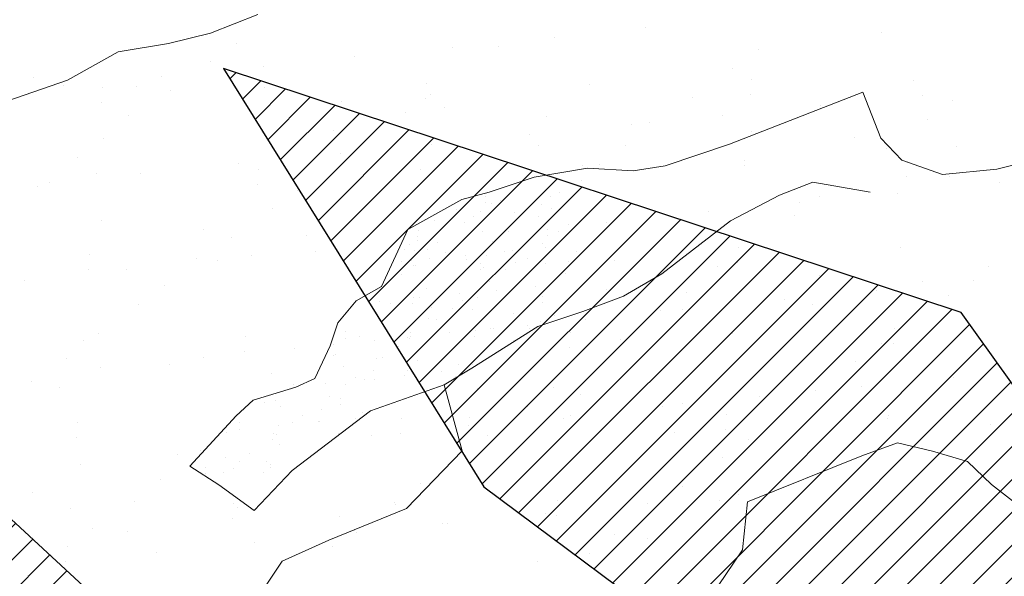
# Model space of a CAD drawing. Units: inches. Extents: x 1986 to 21484, y -1816 to 2016.
# Tile 64 of 85: x 3655.81 to 3662.33, y 1894.988 to 1898.672. Entities that reach past the tile are written whole.
import ezdxf

# ---------------------------------------------------------------- set-up
doc = ezdxf.new("R2010")
doc.units = ezdxf.units.IN
doc.layers.add('L-PLNT', color=84, linetype='Continuous', lineweight=13)
doc.layers.add('vfolhas', color=114, linetype='Continuous', lineweight=5)
doc.layers.add('vfolha2', color=110, linetype='Continuous')
doc.layers.add('vfolhas2', color=102, linetype='Continuous')
pattern_1 = [(45, (-2446.5133113, 50.986076), (-0.004419417382, 0.004419417382), [])]

# ---------------------------------------------------------------- blocks, each defined once
blk = doc.blocks.new('arbusto_PB_verde_grande')
at = {"layer": 'vfolha2'}
h = blk.add_hatch(dxfattribs=at)
h.set_pattern_fill('ANSI31', color=256, scale=0.05, style=0)
h.set_pattern_definition(pattern_1)
h.paths.add_polyline_path([(-0.18963, 0.29704), (-0.08553, 0.20192), (-0.10785, 0.25007), (-0.13202, 0.31865), (-0.25096, 0.48479), (-0.44952, 0.5505), (-0.37946, 0.43789)])
h.paths.add_polyline_path([(0.07911, -0.4071), (0.08214, -0.50631), (0.17255, -0.6355), (0.18428, -0.44151), (0.14904, -0.29177), (0.02625, -0.03934), (0.03527, -0.25376)])
at = {"layer": 'vfolhas'}
h = blk.add_hatch(dxfattribs=at)
h.set_pattern_fill('ANSI31', color=256, scale=0.05, style=0)
h.set_pattern_definition(pattern_1)
h.paths.add_polyline_path([(-0.07279, 0.50669), (-0.18085, 0.65063), (-0.2334, 0.67253), (-0.20712, 0.53176), (-0.10785, 0.25007), (0.02625, -0.03934), (0.00028, 0.09048), (0.00816, 0.16241), (-0.04939, 0.29079)])
h.paths.add_polyline_path([(0.09902, 0.41929), (0.09372, 0.26573), (0.07906, 0.18814), (0.15506, 0.36901), (0.26606, 0.5505), (0.28356, 0.63504), (0.2485, 0.68819), (0.25145, 0.63504), (0.20178, 0.54426)])
h.paths.add_polyline_path([(0.12295, 0.24073), (0.047, 0.06233), (0.02625, -0.03934), (0.11122, 0.04358), (0.18428, 0.09364), (0.27478, 0.19376), (0.3215, 0.25323), (0.44129, 0.38467), (0.47634, 0.57866), (0.41789, 0.45347), (0.28939, 0.30954)])
h.paths.add_polyline_path([(0.58145, -0.03779), (0.70707, 0.01536), (0.78591, 0.04667), (0.74796, 0.06549), (0.62818, 0.08423), (0.52595, 0.09048), (0.39745, 0.04358), (0.02625, -0.03934), (0.25728, -0.03154), (0.43834, -0.0347)])
h.paths.add_polyline_path([(0.52022, -0.03647), (0.43834, -0.0347), (0.25728, -0.03154), (0.02625, -0.03934), (0.17964, -0.08515), (0.53768, -0.13167), (0.69541, -0.15357), (0.78591, -0.07852), (0.70413, -0.10042)])
h.paths.add_polyline_path([(0.27189, -0.21929), (0.14922, -0.14107), (0.02625, -0.03934), (0.15794, -0.31007), (0.29522, -0.42585), (0.41789, -0.49157), (0.56396, -0.56669), (0.5114, -0.48532), (0.39456, -0.34139)])
h.paths.add_polyline_path([(-0.05818, -0.47591), (-0.02312, -0.61984), (0.047, -0.80134), (0.08494, -0.59794), (0.07911, -0.4071), (0.03527, -0.25376), (0.02625, -0.03934), (-0.03773, -0.26001)])
h.paths.add_polyline_path([(-0.24218, 0.14054), (-0.11073, 0.06858), (0.02625, -0.03934), (-0.04235, 0.10871), (-0.21007, 0.23757), (-0.36485, 0.33145), (-0.47874, 0.40341), (-0.54303, 0.46288), (-0.49041, 0.33145), (-0.39408, 0.22192)])
at = {"layer": 'vfolha2'}
for p, q in [((-0.44952, 0.5505), (-0.37946, 0.43789)), ((-0.25096, 0.48479), (-0.44952, 0.5505)), ((-0.13202, 0.31865), (-0.25096, 0.48479)), ((-0.37946, 0.43789), (-0.18963, 0.29704))]:
    blk.add_line(p, q, dxfattribs=at)
at = {"layer": 'vfolhas2'}
blk.add_line((-0.47874, 0.40341), (-0.54303, 0.46288), dxfattribs=at)
blk = doc.blocks.new('PLANT-SHRUB')
for p, q in [((2160.8925, 1877.0609), (2160.9255, 1876.8629)), ((2160.9255, 1876.8629), (2160.9366, 1876.6428)), ((2160.9366, 1876.6428), (2161.0577, 1876.4338)), ((2160.6604, 1876.5701), (2160.6604, 1876.5701)), ((2161.0577, 1876.4338), (2161.1898, 1876.2357)), ((2161.1898, 1876.2357), (2161.4211, 1876.1367)), ((2160.6261, 1876.173), (2160.6261, 1876.173)), ((2161.4211, 1876.1367), (2162.1808, 1875.8396)), ((2162.4231, 1876.0487), (2162.9076, 1876.1587)), ((2161.1081, 1876.0594), (2161.1081, 1876.0594)), ((2161.1297, 1876.0739), (2161.1297, 1876.0739)), ((2162.1808, 1875.8396), (2162.4231, 1876.0487)), ((2159.9502, 1875.7957), (2159.9502, 1875.7957)), ((2160.0857, 1875.7983), (2160.0857, 1875.7983)), ((2161.1081, 1875.8032), (2161.1081, 1875.8032)), ((2160.2751, 1875.7529), (2160.2751, 1875.7529)), ((2160.7604, 1875.7408), (2160.7604, 1875.7408)), ((2162.1875, 1875.7643), (2162.1875, 1875.7643)), ((2160.6867, 1875.6733), (2160.6867, 1875.6733)), ((2160.818, 1875.6814), (2160.818, 1875.6814)), ((2162.3096, 1875.7086), (2162.3096, 1875.7086)), ((2161.026, 1875.654), (2161.026, 1875.654)), ((2161.351, 1875.6112), (2161.351, 1875.6112)), ((2159.4709, 1875.3643), (2159.0745, 1875.5843)), ((2160.3376, 1875.5693), (2160.3376, 1875.5693)), ((2161.8938, 1875.5398), (2161.8938, 1875.5398)), ((2162.8268, 1875.5647), (2162.8268, 1875.5647)), ((2162.1019, 1875.5124), (2162.1019, 1875.5124)), ((2162.4268, 1875.4696), (2162.4268, 1875.4696)), ((2159.5215, 1875.4418), (2159.5215, 1875.4418)), ((2160.6009, 1875.4029), (2160.6009, 1875.4029)), ((2159.7572, 1875.1442), (2159.4709, 1875.3643)), ((2161.6471, 1875.3896), (2161.6471, 1875.3896)), ((2161.9619, 1875.39), (2161.9619, 1875.39)), ((2162.6695, 1875.3945), (2162.6695, 1875.3945)), ((2162.9697, 1875.3981), (2162.9697, 1875.3981)), ((2163.1777, 1875.3708), (2163.1777, 1875.3708)), ((2160.2889, 1875.3088), (2160.2889, 1875.3088)), ((2161.8882, 1875.3225), (2161.8882, 1875.3225)), ((2159.7308, 1875.1827), (2159.7308, 1875.1827)), ((2159.8894, 1874.8912), (2159.7572, 1875.1442)), ((2160.9755, 1875.1805), (2160.9755, 1875.1805)), ((2162.2201, 1875.1782), (2162.2201, 1875.1782)), ((2163.4647, 1875.1759), (2163.4647, 1875.1759)), ((2159.5623, 1875.0754), (2159.5623, 1875.0754)), ((2160.0605, 1875.0282), (2160.0605, 1875.0282)), ((2160.8069, 1875.0731), (2160.8069, 1875.0731)), ((2161.0829, 1875.0331), (2161.0829, 1875.0331)), ((2162.0516, 1875.0708), (2162.0516, 1875.0708)), ((2163.1633, 1875.0392), (2163.1633, 1875.0392)), ((2163.2962, 1875.0686), (2163.2962, 1875.0686)), ((2159.9412, 1874.9901), (2159.9412, 1874.9901)), ((2161.4904, 1874.958), (2161.4904, 1874.958)), ((2162.1624, 1874.9942), (2162.1624, 1874.9942)), ((2163.0897, 1874.9717), (2163.0897, 1874.9717)), ((2163.2085, 1874.9809), (2163.2085, 1874.9809)), ((2159.8676, 1874.9226), (2159.8676, 1874.9226)), ((2159.8896, 1874.6886), (2159.8894, 1874.8912)), ((2160.1867, 1874.9022), (2160.4179, 1874.5941)), ((2159.3737, 1874.8367), (2159.3737, 1874.8367)), ((2159.5817, 1874.8094), (2159.5817, 1874.8094)), ((2159.9066, 1874.7666), (2159.9066, 1874.7666)), ((2159.7682, 1874.385), (2159.8896, 1874.6886)), ((2159.8896, 1874.6886), (2159.8896, 1874.6886)), ((2160.4495, 1874.6951), (2160.4495, 1874.6951)), ((2159.4963, 1874.6717), (2159.4963, 1874.6717)), ((2160.5758, 1874.6328), (2160.5758, 1874.6328)), ((2160.6575, 1874.6677), (2160.6575, 1874.6677)), ((2160.9825, 1874.6249), (2160.9825, 1874.6249)), ((2161.1427, 1874.6394), (2161.1427, 1874.6394)), ((2161.6219, 1874.6195), (2161.6219, 1874.6195)), ((2162.6443, 1874.6244), (2162.6443, 1874.6244)), ((2159.4698, 1874.5581), (2159.4698, 1874.5581)), ((2160.0148, 1874.5685), (2160.0148, 1874.5685)), ((2160.4179, 1874.5941), (2160.6381, 1874.5061)), ((2161.069, 1874.5719), (2161.069, 1874.5719)), ((2161.2594, 1874.5662), (2161.2594, 1874.5662)), ((2161.5253, 1874.5535), (2161.5253, 1874.5535)), ((2162.5041, 1874.5639), (2162.5041, 1874.5639)), ((2162.6919, 1874.6072), (2162.6919, 1874.6072)), ((2163.7238, 1874.5855), (2163.7238, 1874.5855)), ((2163.7487, 1874.5617), (2163.7487, 1874.5617)), ((2160.6381, 1874.5061), (2160.9905, 1874.407)), ((2161.7334, 1874.5261), (2161.7334, 1874.5261)), ((2162.0583, 1874.4833), (2162.0583, 1874.4833)), ((2160.6491, 1874.0329), (2159.7682, 1874.385)), ((2160.9905, 1874.407), (2161.5631, 1874.352)), ((2162.6012, 1874.4118), (2162.6012, 1874.4118)), ((2162.8092, 1874.3845), (2162.8092, 1874.3845)), ((2161.5631, 1874.352), (2161.8494, 1874.286)), ((2163.1157, 1873.9009), (2163.3269, 1874.3016)), ((2163.1341, 1874.3417), (2163.1341, 1874.3417)), ((2163.3269, 1874.3016), (2163.8576, 1874.3262)), ((2163.8576, 1874.3262), (2164.3759, 1874.1289)), ((2160.0353, 1874.2581), (2160.0353, 1874.2581)), ((2161.0577, 1874.263), (2161.0577, 1874.263)), ((2161.8494, 1874.286), (2162.1136, 1874.176)), ((2162.3442, 1874.2886), (2162.3442, 1874.2886)), ((2163.677, 1874.2702), (2163.677, 1874.2702)), ((2163.885, 1874.2428), (2163.885, 1874.2428)), ((2163.8933, 1874.2564), (2163.8933, 1874.2564)), ((2159.4081, 1874.1819), (2159.4081, 1874.1819)), ((2160.6527, 1874.1797), (2160.6527, 1874.1797)), ((2160.6712, 1874.2073), (2160.6712, 1874.2073)), ((2161.8973, 1874.1774), (2161.8973, 1874.1774)), ((2162.1136, 1874.176), (2162.3999, 1874.0439)), ((2162.1372, 1874.2241), (2162.1372, 1874.2241)), ((2162.2705, 1874.2211), (2162.2705, 1874.2211)), ((2163.142, 1874.1751), (2163.142, 1874.1751)), ((2163.1834, 1874.2108), (2163.1834, 1874.2108)), ((2164.2058, 1874.2157), (2164.2058, 1874.2157)), ((2164.2099, 1874.2), (2164.2099, 1874.2)), ((2164.3866, 1874.1729), (2164.3866, 1874.1729)), ((2164.3759, 1874.1289), (2164.6968, 1874.018)), ((2164.6968, 1874.018), (2165.1287, 1874.1166)), ((2160.4841, 1874.0723), (2160.4841, 1874.0723)), ((2161.0566, 1873.8459), (2160.6491, 1874.0329)), ((2161.7288, 1874.07), (2161.7288, 1874.07)), ((2162.2693, 1874.0674), (2162.2693, 1874.0674)), ((2162.3999, 1874.0439), (2162.9065, 1873.9449)), ((2162.9734, 1874.0678), (2162.9734, 1874.0678)), ((2164.218, 1874.0655), (2164.218, 1874.0655)), ((2162.3634, 1874.0292), (2162.3634, 1874.0292)), ((2162.4444, 1873.9883), (2162.4444, 1873.9883)), ((2162.4466, 1874.0183), (2162.4466, 1874.0183)), ((2162.5766, 1874.0012), (2162.5766, 1874.0012)), ((2162.0266, 1873.9128), (2162.0266, 1873.9128)), ((2162.2378, 1873.9208), (2162.2378, 1873.9208)), ((2162.2672, 1873.9478), (2162.2672, 1873.9478)), ((2162.5244, 1873.9119), (2162.5244, 1873.9119)), ((2162.8869, 1873.935), (2162.8869, 1873.935)), ((2162.9065, 1873.9449), (2163.1157, 1873.9009)), ((2163.0223, 1873.911), (2163.0223, 1873.911)), ((2163.1157, 1873.9009), (2163.5892, 1873.6919)), ((2163.5456, 1873.9378), (2163.5456, 1873.9378)), ((2160.3235, 1873.8887), (2160.3235, 1873.8887)), ((2160.5506, 1873.8627), (2160.5506, 1873.8627)), ((2161.2327, 1873.7249), (2161.0566, 1873.8459)), ((2161.5968, 1873.8494), (2161.5968, 1873.8494)), ((2161.8727, 1873.8566), (2161.8727, 1873.8566)), ((2161.9592, 1873.8699), (2161.9592, 1873.8699)), ((2162.2283, 1873.8385), (2162.2283, 1873.8385)), ((2162.457, 1873.869), (2162.457, 1873.869)), ((2162.6192, 1873.8543), (2162.6192, 1873.8543)), ((2162.6372, 1873.8404), (2162.6372, 1873.8404)), ((2162.9549, 1873.868), (2162.9549, 1873.868)), ((2163.472, 1873.8703), (2163.472, 1873.8703)), ((2160.2499, 1873.8212), (2160.2499, 1873.8212)), ((2162.0787, 1873.775), (2162.0787, 1873.775)), ((2162.7184, 1873.7805), (2162.7184, 1873.7805)), ((2162.7478, 1873.8075), (2162.7478, 1873.8075)), ((2163.069, 1873.8249), (2163.069, 1873.8249)), ((2163.6986, 1873.8154), (2163.6986, 1873.8154)), ((2164.7448, 1873.802), (2164.7448, 1873.802)), ((2160.081, 1873.7088), (2160.081, 1873.7088)), ((2161.442, 1873.5048), (2161.2327, 1873.7249)), ((2160.289, 1873.6814), (2160.289, 1873.6814)), ((2161.7857, 1873.6914), (2161.7857, 1873.6914)), ((2161.8689, 1873.6804), (2161.8689, 1873.6804)), ((2161.9396, 1873.6476), (2161.9396, 1873.6476)), ((2161.9989, 1873.6633), (2161.9989, 1873.6633)), ((2162.0026, 1873.6959), (2162.0026, 1873.6959)), ((2162.1402, 1873.6671), (2162.1402, 1873.6671)), ((2162.4344, 1873.6803), (2162.4344, 1873.6803)), ((2162.638, 1873.6662), (2162.638, 1873.6662)), ((2162.8528, 1873.675), (2162.8528, 1873.675)), ((2163.1359, 1873.6653), (2163.1359, 1873.6653)), ((2163.1989, 1873.6402), (2163.1989, 1873.6402)), ((2163.2284, 1873.6672), (2163.2284, 1873.6672)), ((2163.2618, 1873.6769), (2163.2618, 1873.6769)), ((2163.5892, 1873.6919), (2164.2388, 1873.6258)), ((2163.6337, 1873.6644), (2163.6337, 1873.6644)), ((2163.6936, 1873.6614), (2163.6936, 1873.6614)), ((2163.8481, 1873.6543), (2163.8481, 1873.6543)), ((2164.2388, 1873.6258), (2164.6022, 1873.6478)), ((2164.6022, 1873.6478), (2164.6573, 1873.3618)), ((2164.6022, 1873.6478), (2164.6022, 1873.6478)), ((2160.614, 1873.6387), (2160.614, 1873.6387)), ((2161.9101, 1873.6206), (2161.9101, 1873.6206)), ((2162.216, 1873.6347), (2162.216, 1873.6347)), ((2162.2992, 1873.6237), (2162.2992, 1873.6237)), ((2162.4292, 1873.6066), (2162.4292, 1873.6066)), ((2162.5592, 1873.6347), (2162.5592, 1873.6347)), ((2162.6463, 1873.578), (2162.6463, 1873.578)), ((2164.7471, 1873.587), (2164.7471, 1873.587)), ((2160.9366, 1873.5654), (2160.9366, 1873.5654)), ((2161.1568, 1873.5672), (2161.1568, 1873.5672)), ((2161.3649, 1873.5398), (2161.3649, 1873.5398)), ((2161.525, 1873.5379), (2161.525, 1873.5379)), ((2161.7997, 1873.5358), (2161.7997, 1873.5358)), ((2161.8975, 1873.5125), (2161.8975, 1873.5125)), ((2162.1813, 1873.5631), (2162.1813, 1873.5631)), ((2162.2182, 1873.5304), (2162.2182, 1873.5304)), ((2162.3953, 1873.5116), (2162.3953, 1873.5116)), ((2162.6272, 1873.5324), (2162.6272, 1873.5324)), ((2162.7296, 1873.5671), (2162.7296, 1873.5671)), ((2162.8595, 1873.55), (2162.8595, 1873.55)), ((2162.8932, 1873.5107), (2162.8932, 1873.5107)), ((2163.0589, 1873.5168), (2163.0589, 1873.5168)), ((2163.0767, 1873.5214), (2163.0767, 1873.5214)), ((2163.1599, 1873.5104), (2163.1599, 1873.5104)), ((2163.391, 1873.5098), (2163.391, 1873.5098)), ((2163.4259, 1873.5609), (2163.4259, 1873.5609)), ((2163.4774, 1873.5115), (2163.4774, 1873.5115)), ((2163.709, 1873.5269), (2163.709, 1873.5269)), ((2163.8864, 1873.5134), (2163.8864, 1873.5134)), ((2164.3287, 1873.514), (2164.3287, 1873.514)), ((2164.6705, 1873.5586), (2164.6705, 1873.5586)), ((2164.6734, 1873.5195), (2164.6734, 1873.5195)), ((2161.0325, 1873.4929), (2161.0325, 1873.4929)), ((2161.7393, 1873.3068), (2161.442, 1873.5048)), ((2161.4513, 1873.4704), (2161.4513, 1873.4704)), ((2161.6898, 1873.497), (2161.6898, 1873.497)), ((2161.751, 1873.4748), (2161.751, 1873.4748)), ((2161.8301, 1873.4695), (2161.8301, 1873.4695)), ((2162.112, 1873.454), (2162.112, 1873.454)), ((2162.3279, 1873.4686), (2162.3279, 1873.4686)), ((2162.3907, 1873.4803), (2162.3907, 1873.4803)), ((2162.4202, 1873.5073), (2162.4202, 1873.5073)), ((2162.8258, 1873.4677), (2162.8258, 1873.4677)), ((2163.0398, 1873.4944), (2163.0398, 1873.4944)), ((2163.0742, 1873.5058), (2163.0742, 1873.5058)), ((2163.2899, 1873.4933), (2163.2899, 1873.4933)), ((2163.3236, 1873.4668), (2163.3236, 1873.4668)), ((2163.507, 1873.4647), (2163.507, 1873.4647)), ((2163.5902, 1873.4538), (2163.5902, 1873.4538)), ((2163.6795, 1873.4999), (2163.6795, 1873.4999)), ((2163.8215, 1873.4659), (2163.8215, 1873.4659)), ((2163.8889, 1873.5089), (2163.8889, 1873.5089)), ((2164.1806, 1873.4456), (2164.1806, 1873.4456)), ((2164.3182, 1873.4979), (2164.3182, 1873.4979)), ((2164.3193, 1873.465), (2164.3193, 1873.465)), ((2164.3867, 1873.508), (2164.3867, 1873.508)), ((2161.9925, 1873.3878), (2161.9925, 1873.3878)), ((2162.2327, 1873.4255), (2162.2327, 1873.4255)), ((2162.4407, 1873.3982), (2162.4407, 1873.3982)), ((2163.1582, 1873.4407), (2163.1582, 1873.4407)), ((2163.7202, 1873.4367), (2163.7202, 1873.4367)), ((2163.9373, 1873.4081), (2163.9373, 1873.4081)), ((2164.0205, 1873.3971), (2164.0205, 1873.3971)), ((2164.1505, 1873.38), (2164.1505, 1873.38)), ((2164.1896, 1873.3866), (2164.1896, 1873.3866)), ((2165.2601, 1873.4067), (2165.2601, 1873.4067)), ((2162.2316, 1873.3345), (2162.2316, 1873.3345)), ((2162.4243, 1873.3723), (2162.4243, 1873.3723)), ((2162.7656, 1873.3554), (2162.7656, 1873.3554)), ((2162.8428, 1873.3669), (2162.8428, 1873.3669)), ((2162.8713, 1873.3399), (2162.8713, 1873.3399)), ((2162.9007, 1873.3669), (2162.9007, 1873.3669)), ((2163.2517, 1873.3689), (2163.2517, 1873.3689)), ((2163.5204, 1873.3541), (2163.5204, 1873.3541)), ((2163.6835, 1873.3533), (2163.6835, 1873.3533)), ((2164.102, 1873.348), (2164.102, 1873.348)), ((2164.1601, 1873.3596), (2164.1601, 1873.3596)), ((2164.3677, 1873.3514), (2164.3677, 1873.3514)), ((2164.4509, 1873.3405), (2164.4509, 1873.3405)), ((2164.5109, 1873.35), (2164.5109, 1873.35)), ((2164.5808, 1873.3234), (2164.5808, 1873.3234)), ((2164.6573, 1873.3618), (2164.7123, 1873.1417)), ((2162.0256, 1873.1747), (2161.7393, 1873.3068)), ((2161.8515, 1873.2688), (2161.8515, 1873.2688)), ((2162.0111, 1873.2668), (2162.0111, 1873.2668)), ((2162.5089, 1873.2659), (2162.5089, 1873.2659)), ((2163.0068, 1873.265), (2163.0068, 1873.265)), ((2163.3085, 1873.2839), (2163.3085, 1873.2839)), ((2163.7103, 1873.2848), (2163.4901, 1873.1967)), ((2163.5046, 1873.2641), (2163.5046, 1873.2641)), ((2163.5165, 1873.2565), (2163.5165, 1873.2565)), ((2163.8424, 1873.2407), (2163.7103, 1873.2848)), ((2164.0025, 1873.2632), (2164.0025, 1873.2632)), ((2164.5003, 1873.2622), (2164.5003, 1873.2622)), ((2162.0686, 1873.2402), (2162.0686, 1873.2402)), ((2162.0925, 1873.207), (2162.0925, 1873.207)), ((2162.1518, 1873.2292), (2162.1518, 1873.2292)), ((2162.2081, 1873.2224), (2162.2081, 1873.2224)), ((2162.2818, 1873.2121), (2162.2818, 1873.2121)), ((2162.6171, 1873.2243), (2162.6171, 1873.2243)), ((2162.7122, 1873.1941), (2162.7122, 1873.1941)), ((2162.7264, 1873.1872), (2162.7264, 1873.1872)), ((2163.0489, 1873.2088), (2163.0489, 1873.2088)), ((2163.4901, 1873.1967), (2163.3469, 1873.1197)), ((2163.3519, 1873.1996), (2163.3519, 1873.1996)), ((2163.3813, 1873.2266), (2163.3813, 1873.2266)), ((2163.4673, 1873.2034), (2163.4673, 1873.2034)), ((2163.8414, 1873.2137), (2163.8414, 1873.2137)), ((2164.1067, 1873.1087), (2163.8424, 1873.2407)), ((2164.001, 1873.2138), (2164.001, 1873.2138)), ((2164.3081, 1873.1898), (2164.3081, 1873.1898)), ((2164.6407, 1873.2193), (2164.6407, 1873.2193)), ((2164.6702, 1873.2463), (2164.6702, 1873.2463)), ((2161.5745, 1873.1766), (2161.5745, 1873.1766)), ((2162.1907, 1873.0867), (2162.0256, 1873.1747)), ((2162.063, 1873.18), (2162.063, 1873.18)), ((2162.4989, 1873.1835), (2162.4989, 1873.1835)), ((2162.5822, 1873.1726), (2162.5822, 1873.1726)), ((2162.9725, 1873.1417), (2162.5871, 1872.9877)), ((2162.6528, 1873.1197), (2162.6528, 1873.1197)), ((2162.7121, 1873.1555), (2162.7121, 1873.1555)), ((2162.8192, 1873.1743), (2162.8192, 1873.1743)), ((2162.9293, 1873.1269), (2162.9293, 1873.1269)), ((2162.9725, 1873.1417), (2162.9725, 1873.1417)), ((2163.1597, 1873.0977), (2162.9725, 1873.1417)), ((2163.3469, 1873.1197), (2163.1597, 1873.0977)), ((2164.0638, 1873.1721), (2164.0638, 1873.1721)), ((2164.7123, 1873.1417), (2164.2609, 1873.1087)), ((2164.2756, 1873.155), (2164.2756, 1873.155)), ((2164.3843, 1873.1423), (2164.3843, 1873.1423)), ((2164.7123, 1873.1417), (2164.7123, 1873.1417)), ((2165.3084, 1873.1698), (2165.3084, 1873.1698)), ((2160.5254, 1873.0926), (2160.5254, 1873.0926)), ((2161.0535, 1873.1059), (2161.0535, 1873.1059)), ((2161.406, 1873.0692), (2161.406, 1873.0692)), ((2161.5716, 1873.0793), (2161.5716, 1873.0793)), ((2162.5871, 1872.9877), (2162.1907, 1873.0867)), ((2162.2662, 1873.1112), (2162.2662, 1873.1112)), ((2162.4142, 1873.0642), (2162.4142, 1873.0642)), ((2162.5731, 1873.0667), (2162.5731, 1873.0667)), ((2162.594, 1873.0842), (2162.594, 1873.0842)), ((2162.6506, 1873.0669), (2162.6506, 1873.0669)), ((2162.6967, 1873.0674), (2162.6967, 1873.0674)), ((2162.7641, 1873.1103), (2162.7641, 1873.1103)), ((2163.8953, 1873.0647), (2163.8953, 1873.0647)), ((2164.2609, 1873.1087), (2164.1067, 1873.1087)), ((2164.5923, 1873.1149), (2164.5923, 1873.1149)), ((2164.9173, 1873.0721), (2164.9173, 1873.0721)), ((2165.1399, 1873.0624), (2165.1399, 1873.0624)), ((2162.5436, 1873.0397), (2162.5436, 1873.0397)), ((2163.6734, 1873.0453), (2163.6734, 1873.0453)), ((2164.7196, 1873.032), (2164.7196, 1873.032)), ((2165.4601, 1873.0006), (2165.4601, 1873.0006)), ((2165.742, 1873.0369), (2165.742, 1873.0369)), ((2165.6682, 1872.9733), (2165.6682, 1872.9733)), ((2165.9931, 1872.9305), (2165.9931, 1872.9305)), ((2163.9279, 1872.8364), (2163.9279, 1872.8364)), ((2165.4771, 1872.8042), (2165.4771, 1872.8042)), ((2162.255, 1872.7551), (2162.255, 1872.7551)), ((2163.8542, 1872.7689), (2163.8542, 1872.7689)), ((2161.0074, 1872.7228), (2161.0074, 1872.7228)), ((2162.0868, 1872.6839), (2162.0868, 1872.6839)), ((2163.133, 1872.6706), (2163.133, 1872.6706)), ((2164.1554, 1872.6755), (2164.1554, 1872.6755)), ((2165.2349, 1872.6366), (2165.2349, 1872.6366)), ((2161.8585, 1872.5623), (2161.8585, 1872.5623)), ((2163.1031, 1872.56), (2163.1031, 1872.56)), ((2164.3478, 1872.5578), (2164.3478, 1872.5578)), ((2165.5924, 1872.5555), (2165.5924, 1872.5555)), ((2161.3213, 1872.5107), (2161.3213, 1872.5107)), ((2165.1294, 1872.4856), (2165.1294, 1872.4856)), ((2161.8642, 1872.4393), (2161.8642, 1872.4393)), ((2161.9073, 1872.4365), (2161.9073, 1872.4365)), ((2162.0722, 1872.4119), (2162.0722, 1872.4119)), ((2163.4564, 1872.4044), (2163.4564, 1872.4044)), ((2165.0557, 1872.4181), (2165.0557, 1872.4181)), ((2161.8336, 1872.369), (2161.8336, 1872.369)), ((2162.3971, 1872.3691), (2162.3971, 1872.3691)), ((2161.5464, 1872.3092), (2161.5464, 1872.3092)), ((2162.5688, 1872.3141), (2162.5688, 1872.3141)), ((2162.94, 1872.2976), (2162.94, 1872.2976)), ((2163.6483, 1872.2752), (2163.6483, 1872.2752)), ((2163.148, 1872.2702), (2163.148, 1872.2702)), ((2163.4729, 1872.2275), (2163.4729, 1872.2275)), ((2164.6944, 1872.2619), (2164.6944, 1872.2619)), ((2162.4964, 1872.1735), (2162.4964, 1872.1735)), ((2163.741, 1872.1712), (2163.741, 1872.1712)), ((2164.0158, 1872.156), (2164.0158, 1872.156)), ((2164.9856, 1872.169), (2164.9856, 1872.169)), ((2163.1087, 1872.0857), (2163.1087, 1872.0857)), ((2164.2238, 1872.1286), (2164.2238, 1872.1286)), ((2164.5488, 1872.0858), (2164.5488, 1872.0858)), ((2162.3278, 1872.0661), (2162.3278, 1872.0661)), ((2163.0351, 1872.0182), (2163.0351, 1872.0182)), ((2163.5725, 1872.0639), (2163.5725, 1872.0639)), ((2164.6579, 1872.0536), (2164.6579, 1872.0536)), ((2164.8171, 1872.0616), (2164.8171, 1872.0616)), ((2165.0916, 1872.0143), (2165.0916, 1872.0143)), ((2162.0617, 1871.9138), (2162.0617, 1871.9138)), ((2163.1078, 1871.9005), (2163.1078, 1871.9005)), ((2164.1302, 1871.9054), (2164.1302, 1871.9054)), ((2164.3102, 1871.735), (2164.3102, 1871.735)), ((2162.6373, 1871.6537), (2162.6373, 1871.6537)), ((2164.2365, 1871.6675), (2164.2365, 1871.6675)), ((2162.7803, 1871.5592), (2162.7803, 1871.5592)), ((2164.025, 1871.557), (2164.025, 1871.557)), ((2162.5436, 1871.544), (2162.5436, 1871.544)), ((2163.6231, 1871.5051), (2163.6231, 1871.5051)), ((2164.6693, 1871.4918), (2164.6693, 1871.4918)), ((2162.5715, 1871.3113), (2162.5715, 1871.3113)), ((2163.8387, 1871.3029), (2163.8387, 1871.3029)), ((2162.3387, 1871.269), (2162.6507, 1871.1444)), ((2162.7795, 1871.2839), (2162.7795, 1871.2839)), ((2163.1045, 1871.2412), (2163.1045, 1871.2412)), ((2163.4182, 1871.1704), (2163.4182, 1871.1704)), ((2163.6473, 1871.1697), (2163.6473, 1871.1697)), ((2162.6507, 1871.1444), (2162.9002, 1871.0041)), ((2163.0827, 1871.1304), (2163.0827, 1871.1304)), ((2163.8554, 1871.1423), (2163.8554, 1871.1423)), ((2164.1051, 1871.1353), (2164.1051, 1871.1353)), ((2164.1803, 1871.0995), (2164.1803, 1871.0995)), ((2163.2497, 1871.063), (2163.2497, 1871.063)), ((2162.9002, 1871.0041), (2163.1809, 1870.8171)), ((2163.491, 1870.9843), (2163.491, 1870.9843)), ((2163.4173, 1870.9168), (2163.4173, 1870.9168)), ((2163.1809, 1870.8171), (2163.5552, 1870.7236)), ((2163.1809, 1870.8171), (2163.1809, 1870.8171)), ((2163.5552, 1870.7236), (2164.0075, 1870.521)), ((2163.5979, 1870.735), (2163.5979, 1870.735)), ((2163.7022, 1870.5561), (2163.7022, 1870.5561))]:
    blk.add_line(p, q)

msp = doc.modelspace()

# ---------------------------------------------------------------- block references
at = {"layer": 'L-PLNT', "rotation": 223.1883365522388}
msp.add_blockref('PLANT-SHRUB', (3953.27, 4742.9646), dxfattribs=at)
at = {"layer": 'L-PLNT', "xscale": 24.60366729364114, "yscale": 24.60366729364114, "zscale": 24.60366729364114}
msp.add_blockref('arbusto_PB_verde_grande', (3668.2184, 1884.8051), dxfattribs=at)

doc.saveas('drawing.dxf')
